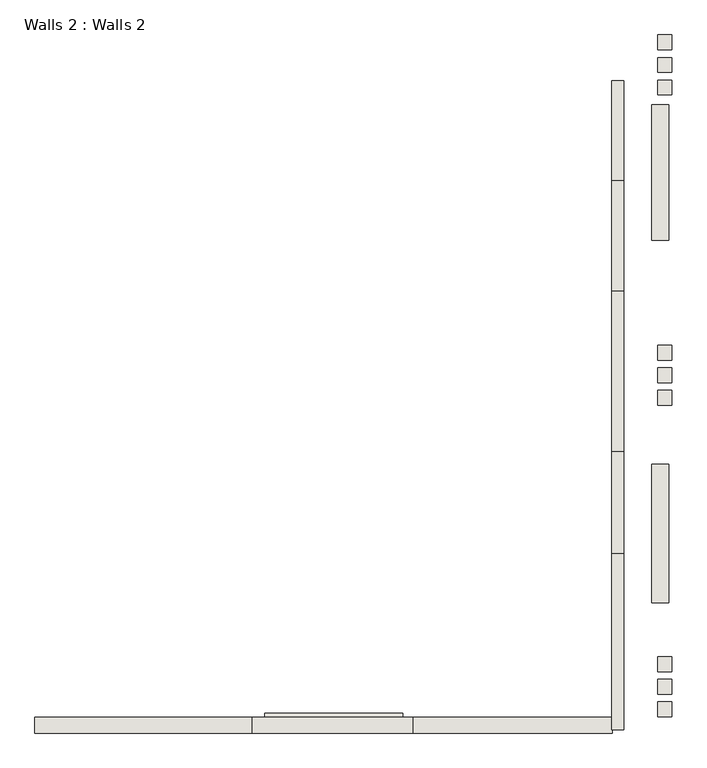
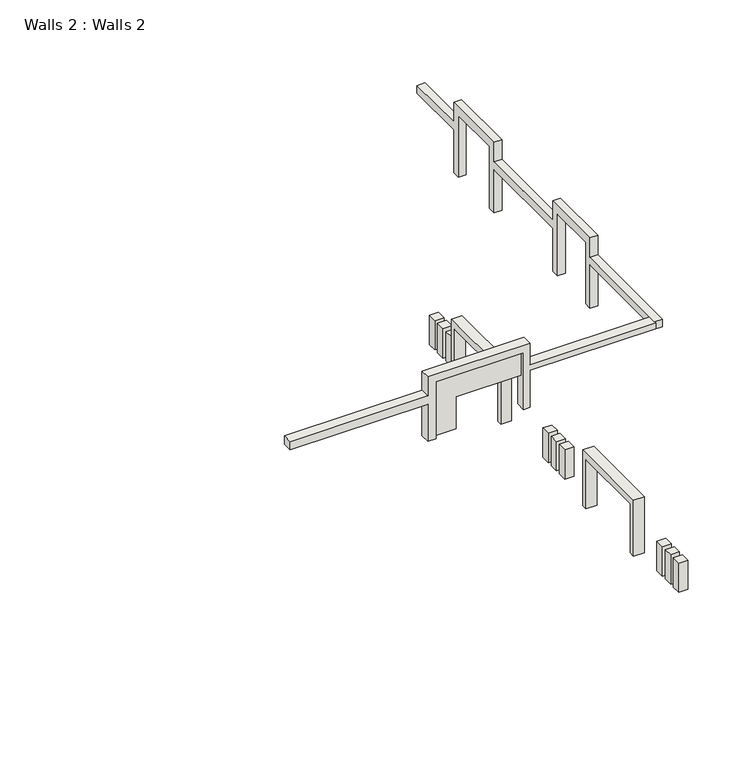
"""IFC4 building model written with IfcOpenShell, lengths in millimetres: wall geometry, Walls 2 : Walls 2."""

from ifc_helpers import new_model, si_unit, frame, origin, place, context, project, spatial, polyline, outline, extrude, source, transform, mapped, element, save


def walls_2_walls_2_7a041f15(model_context):
    return source(origin(), model_context, "Body", "SweptSolid", [
        extrude(outline(polyline([(3353.6074298, -3256.5259649), (3353.6074298, -3523.2259649), (3099.6074298, -3523.2259649), (3099.6074298, -3256.5259649), (3353.6074298, -3256.5259649)])), frame((0.0, 0.0, 576.2769048), z_axis=(0.0, 0.0, 1.0), x_axis=(1.0, 0.0, 0.0)), (0.0, 0.0, 1.0), 881.8439498),
        extrude(outline(polyline([(3353.6074298, -2850.1259649), (3353.6074298, -3116.8259649), (3099.6074298, -3116.8259649), (3099.6074298, -2850.1259649), (3353.6074298, -2850.1259649)])), frame((0.0, 0.0, 576.2769048), z_axis=(0.0, 0.0, 1.0), x_axis=(1.0, 0.0, 0.0)), (0.0, 0.0, 1.0), 881.8439498),
        extrude(outline(polyline([(3353.6074298, -2443.7259649), (3353.6074298, -2710.4259649), (3099.6074298, -2710.4259649), (3099.6074298, -2443.7259649), (3353.6074298, -2443.7259649)])), frame((0.0, 0.0, 576.2769048), z_axis=(0.0, 0.0, 1.0), x_axis=(1.0, 0.0, 0.0)), (0.0, 0.0, 1.0), 881.8439498),
        extrude(outline(polyline([(3353.6074298, 2356.8740351), (3353.6074298, 2090.1740351), (3099.6074298, 2090.1740351), (3099.6074298, 2356.8740351), (3353.6074298, 2356.8740351)])), frame((0.0, 0.0, 576.2769048), z_axis=(0.0, 0.0, 1.0), x_axis=(1.0, 0.0, 0.0)), (0.0, 0.0, 1.0), 881.8439498),
        extrude(outline(polyline([(3353.6074298, 2763.2740351), (3353.6074298, 2496.5740351), (3099.6074298, 2496.5740351), (3099.6074298, 2763.2740351), (3353.6074298, 2763.2740351)])), frame((0.0, 0.0, 576.2769048), z_axis=(0.0, 0.0, 1.0), x_axis=(1.0, 0.0, 0.0)), (0.0, 0.0, 1.0), 881.8439498),
        extrude(outline(polyline([(3353.6074298, 3169.6740351), (3353.6074298, 2902.9740351), (3099.6074298, 2902.9740351), (3099.6074298, 3169.6740351), (3353.6074298, 3169.6740351)])), frame((0.0, 0.0, 576.2769048), z_axis=(0.0, 0.0, 1.0), x_axis=(1.0, 0.0, 0.0)), (0.0, 0.0, 1.0), 881.8439498),
        extrude(outline(polyline([(3353.6074298, 7944.8740351), (3353.6074298, 7678.1740351), (3099.6074298, 7678.1740351), (3099.6074298, 7944.8740351), (3353.6074298, 7944.8740351)])), frame((0.0, 0.0, 576.2769048), z_axis=(0.0, 0.0, 1.0), x_axis=(1.0, 0.0, 0.0)), (0.0, 0.0, 1.0), 881.8439498),
        extrude(outline(polyline([(3353.6074298, 8351.2740351), (3353.6074298, 8084.5740351), (3099.6074298, 8084.5740351), (3099.6074298, 8351.2740351), (3353.6074298, 8351.2740351)])), frame((0.0, 0.0, 576.2769048), z_axis=(0.0, 0.0, 1.0), x_axis=(1.0, 0.0, 0.0)), (0.0, 0.0, 1.0), 881.8439498),
        extrude(outline(polyline([(3353.6074298, 8757.6740351), (3353.6074298, 8490.9740351), (3099.6074298, 8490.9740351), (3099.6074298, 8757.6740351), (3353.6074298, 8757.6740351)])), frame((0.0, 0.0, 576.2769048), z_axis=(0.0, 0.0, 1.0), x_axis=(1.0, 0.0, 0.0)), (0.0, 0.0, 1.0), 881.8439498),
        extrude(outline(polyline([(-1465.8259649, 457.2), (-1465.8259649, 2133.6), (1023.3740351, 2133.6), (1023.3740351, 457.2), (870.9740351, 457.2), (870.9740351, 1930.4), (-1313.4259649, 1930.4), (-1313.4259649, 457.2), (-1465.8259649, 457.2)])), frame((2998.0074298, 0.0, 0.0), z_axis=(1.0, 0.0, 0.0), x_axis=(0.0, 1.0, 0.0)), (0.0, 0.0, 1.0), 304.8),
        extrude(outline(polyline([(5061.4786759, 457.2), (5061.4786759, 2133.6), (7499.8786759, 2133.6), (7499.8786759, 457.2), (7347.4786759, 457.2), (7347.4786759, 1930.4), (5213.8786759, 1930.4), (5213.8786759, 457.2), (5061.4786759, 457.2)])), frame((2998.0074298, 0.0, 0.0), z_axis=(1.0, 0.0, 0.0), x_axis=(0.0, 1.0, 0.0)), (0.0, 0.0, 1.0), 304.8),
        extrude(outline(polyline([(-576.8259649, 9144.0), (-576.8259649, 9731.3133194), (1251.9740351, 9731.3133194), (1251.9740351, 9144.0), (4147.5740351, 9144.0), (4147.5740351, 9731.3133194), (6128.7740351, 9731.3133194), (6128.7740351, 9144.0), (7932.1740351, 9144.0), (7932.1740351, 8915.4), (6128.7740351, 8915.4), (6128.7740351, 7620.0), (5900.1740351, 7620.0), (5900.1740351, 9474.2), (4376.1740351, 9474.2), (4376.1740351, 7620.0), (4147.5740351, 7620.0), (4147.5740351, 8915.4), (1251.9740351, 8915.4), (1251.9740351, 7620.0), (1023.3740351, 7620.0), (1023.3740351, 9474.2), (-373.6259649, 9474.2), (-373.6259649, 8915.4), (-373.6259649, 7620.0), (-576.8259649, 7620.0), (-576.8259649, 8915.4), (-3758.9075805, 8915.4), (-3758.9075805, 9144.0), (-576.8259649, 9144.0)])), frame((2272.4271302, 0.0, 0.0), z_axis=(1.0, 0.0, 0.0), x_axis=(0.0, 1.0, 0.0)), (0.0, 0.0, 1.0), 220.7761234),
        extrude(outline(polyline([(9556.7547619, -1486.7728698), (9556.7547619, -3975.9728698), (7854.9547619, -3975.9728698), (7854.9547619, -3340.9728698), (8820.1547619, -3340.9728698), (8820.1547619, -1486.7728698), (9556.7547619, -1486.7728698)])), frame((0.0, -3701.0259649, 0.0), z_axis=(0.0, 1.0, 0.0), x_axis=(0.0, 0.0, 1.0)), (0.0, 0.0, 1.0), 236.8657924),
        extrude(outline(polyline([(9212.8470483, -4204.5728698), (9212.8470483, -8116.1728698), (8966.2, -8116.1728698), (8966.2, -4204.5728698), (7854.9547619, -4204.5728698), (7854.9547619, -3975.9728698), (9556.7547619, -3975.9728698), (9556.7547619, -1486.7728698), (7854.9547619, -1486.7728698), (7854.9547619, -1308.9728698), (8966.2, -1308.9728698), (8966.2, 2282.3662071), (9144.0, 2282.3662071), (9144.0, -1308.9728698), (9785.7694166, -1308.9728698), (9785.7694166, -4204.5728698), (9212.8470483, -4204.5728698)])), frame((0.0, -3817.2037109, 0.0), z_axis=(0.0, 1.0, 0.0), x_axis=(0.0, 0.0, 1.0)), (0.0, 0.0, 1.0), 281.2777461),
    ])


if __name__ == "__main__":
    model = new_model("IFC4")
    model_context = context("Model", 3, world=origin())
    ifc_project = project(units=[si_unit("LENGTHUNIT", "METRE", prefix="MILLI")], contexts=[model_context])
    site = spatial("IfcSite", under=ifc_project)
    building = spatial("IfcBuilding", under=site)
    placement = place(None, origin())
    walls_2_walls_2_shape = walls_2_walls_2_7a041f15(model_context)
    element("IfcWall", 1, ObjectType="Walls 2 : Walls 2", at=placement, inside=building, context=model_context, shape_type="MappedRepresentation", body=[
        mapped(walls_2_walls_2_shape, transform((0.0, 0.0, 0.0), x_axis=(1.0, 0.0, 0.0), y_axis=(0.0, 1.0, 0.0), z_axis=(0.0, 0.0, 1.0))),
    ])
    save(model, "model.ifc")

# Revit data of these elements
# Element 1 (IfcWall, "Walls 2 : Walls 2")
#   Materials on its faces: "Default Wall"
# Materials
#   "Default Wall": colour RGB 128 128 128, transparency 0
